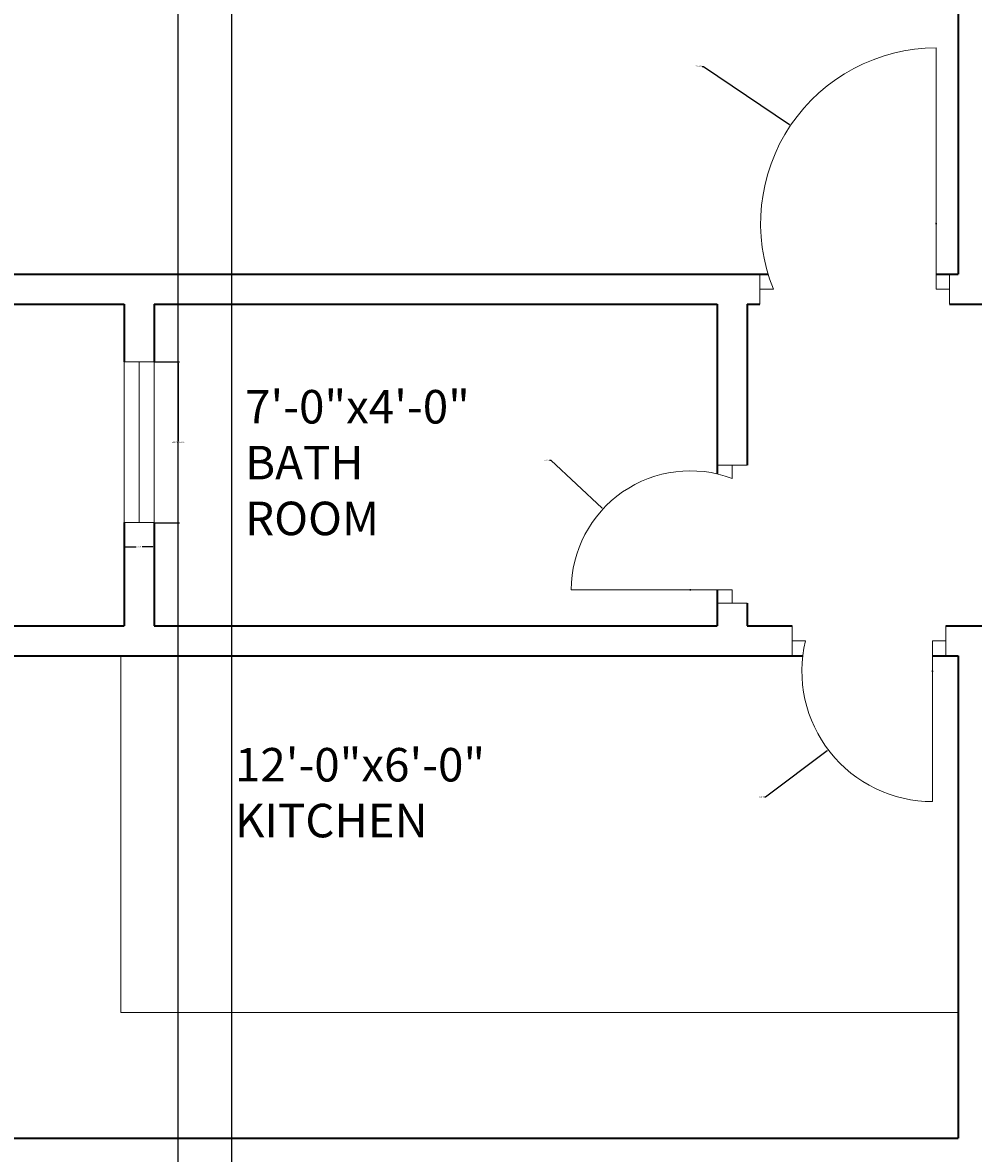
# Model space of a CAD drawing. Units: inches. Extents: x 2163 to 2982, y 1024 to 2288.
# Tile 11 of 22: x 2306 to 2448, y 1885 to 2054. Entities that reach past the tile are written whole.
import ezdxf

# ---------------------------------------------------------------- set-up
doc = ezdxf.new("R2010")
doc.units = ezdxf.units.IN
for name, color, linetype, lineweight in [('A-ANNO-DIMS', 2, 'Continuous', 18), ('A-AREA-IDEN', 7, 'Continuous', 18), ('A-DOOR', 11, 'Continuous', 18), ('A-FLOR-FIXT', 9, 'Continuous', 18), ('A-GLAZ', 161, 'Continuous', 18), ('A-WALL', 7, 'Continuous', 35)]:
    doc.layers.add(name, color=color, linetype=linetype, lineweight=lineweight)
doc.styles.get("Standard").update_dxf_attribs({"font": 'arial.ttf'})
doc.dimstyles.get("Standard").update_dxf_attribs({"dimtxt": 0.18, "dimasz": 0.18, "dimexe": 0.18, "dimexo": 0.0625, "dimgap": 0.09, "dimtad": 0, "dimtih": 1, "dimtoh": 1, "dimdec": 4, "dimzin": 0, "dimdsep": 46, "dimtxsty": 'Standard', "dimcen": 0.09, "dimadec": 0, "dimazin": 0, "dimtfac": 1, "dimtdec": 4, "dimtofl": 0, "dimtmove": 0, "dimatfit": 3, "dimfxl": 1, "dimtolj": 1, "dimtzin": 0, "dimarcsym": 0})

# ---------------------------------------------------------------- blocks, each defined once
blk = doc.blocks.new('WIN-24')
for p, q in [((0, 24), (4.5, 24)), ((0, 24), (0, 0)), ((4.5, 24), (2.25, 24)), ((2.25, 24), (2.25, 0)), ((4.5, 24), (4.5, 0)), ((2.25, 0), (0, 0)), ((0, 0), (4.5, 0))]:
    blk.add_line(p, q)
blk = doc.blocks.new('*D11')
at = {"layer": 'A-ANNO-DIMS', "color": 0, "lineweight": -2, "transparency": 16777216}
for p, q in [((2325.9, 2003.16), (2329.62, 2003.16)), ((2329.44, 2002.98), (2329.44, 1991.35)), ((2329.44, 1979.34), (2329.44, 1990.98)), ((2325.9, 1979.16), (2329.62, 1979.16))]:
    blk.add_line(p, q, dxfattribs=at)
at = {"layer": 'A-ANNO-DIMS', "color": 0, "transparency": 16777216}
for points in [[(2329.41, 2002.98), (2329.47, 2002.98), (2329.44, 2003.16)], [(2329.41, 1979.34), (2329.47, 1979.34), (2329.44, 1979.16)]]:
    blk.add_solid(points, dxfattribs=at)
at = {"layer": 'Defpoints', "color": 0, "transparency": 16777216}
for p in [(2325.84, 2003.16), (2329.44, 2003.16), (2325.84, 1979.16)]:
    blk.add_point(p, dxfattribs=at)
at = {"layer": 'A-ANNO-DIMS', "color": 0, "transparency": 16777216, "insert": (2329.44, 1991.16), "char_height": 0.18, "attachment_point": 5}
blk.add_mtext('\\A1;WINDOW 24 TYP.', dxfattribs=at)
blk = doc.blocks.new('*D12')
at = {"layer": 'A-ANNO-DIMS', "color": 0, "lineweight": -2, "transparency": 16777216}
for p, q in [((2321.34, 1979.1), (2321.34, 1975.38)), ((2325.84, 1979.1), (2325.84, 1975.38)), ((2321.52, 1975.56), (2323.13, 1975.56)), ((2325.66, 1975.56), (2324.05, 1975.56))]:
    blk.add_line(p, q, dxfattribs=at)
at = {"layer": 'A-ANNO-DIMS', "color": 0, "transparency": 16777216}
for points in [[(2321.52, 1975.59), (2321.52, 1975.53), (2321.34, 1975.56)], [(2325.66, 1975.59), (2325.66, 1975.53), (2325.84, 1975.56)]]:
    blk.add_solid(points, dxfattribs=at)
at = {"layer": 'Defpoints', "color": 0, "transparency": 16777216}
for p in [(2321.34, 1979.16), (2325.84, 1979.16), (2325.84, 1975.56)]:
    blk.add_point(p, dxfattribs=at)
at = {"layer": 'A-ANNO-DIMS', "color": 0, "transparency": 16777216, "insert": (2323.59, 1975.56), "char_height": 0.18, "attachment_point": 5}
blk.add_mtext('\\A1;5 TYP.', dxfattribs=at)
blk = doc.blocks.new('*D29')
at = {"layer": 'A-ANNO-DIMS', "color": 0, "lineweight": -2, "transparency": 16777216}
for p, q in [((2285.34, 1738.83), (2285.34, 2288.1)), ((2285.52, 2287.92), (2576.05, 2287.92)), ((2867.16, 2287.92), (2576.63, 2287.92)), ((2867.34, 2229.33), (2867.34, 2288.1))]:
    blk.add_line(p, q, dxfattribs=at)
at = {"layer": 'A-ANNO-DIMS', "color": 0, "transparency": 16777216}
for points in [[(2285.52, 2287.95), (2285.52, 2287.89), (2285.34, 2287.92)], [(2867.16, 2287.95), (2867.16, 2287.89), (2867.34, 2287.92)]]:
    blk.add_solid(points, dxfattribs=at)
at = {"layer": 'Defpoints', "color": 0, "transparency": 16777216}
for p in [(2867.34, 2287.92), (2867.34, 2229.27), (2285.34, 1738.77)]:
    blk.add_point(p, dxfattribs=at)
at = {"layer": 'A-ANNO-DIMS', "color": 0, "transparency": 16777216, "insert": (2576.34, 2287.92), "char_height": 0.18, "attachment_point": 5}
blk.add_mtext('\\A1;582', dxfattribs=at)
blk = doc.blocks.new('*D38')
at = {"layer": 'A-ANNO-DIMS', "color": 0, "lineweight": -2, "transparency": 16777216}
for p, q in [((2329.44, 1734.33), (2329.44, 2288.1)), ((2329.62, 2287.92), (2333.29, 2287.92)), ((2337.26, 2287.92), (2333.59, 2287.92)), ((2337.44, 1734.33), (2337.44, 2288.1))]:
    blk.add_line(p, q, dxfattribs=at)
at = {"layer": 'A-ANNO-DIMS', "color": 0, "transparency": 16777216}
for points in [[(2329.62, 2287.95), (2329.62, 2287.89), (2329.44, 2287.92)], [(2337.26, 2287.95), (2337.26, 2287.89), (2337.44, 2287.92)]]:
    blk.add_solid(points, dxfattribs=at)
at = {"layer": 'Defpoints', "color": 0, "transparency": 16777216}
for p in [(2337.44, 2287.92), (2329.44, 1734.27), (2337.44, 1734.27)]:
    blk.add_point(p, dxfattribs=at)
at = {"layer": 'A-ANNO-DIMS', "color": 0, "transparency": 16777216, "insert": (2333.44, 2287.92), "char_height": 0.18, "attachment_point": 5}
blk.add_mtext('\\A1;8', dxfattribs=at)
blk = doc.blocks.new('*D53')
at = {"layer": 'A-ANNO-DIMS', "color": 0, "lineweight": -2, "transparency": 16777216}
for p, q in [((2407.61, 2047.27), (2407.79, 2047.27)), ((2407.79, 2047.27), (2420.67, 2038.58)), ((2442.45, 2023.82), (2442.63, 2023.82)), ((2442.54, 2023.73), (2442.54, 2023.91))]:
    blk.add_line(p, q, dxfattribs=at)
at = {"layer": 'A-ANNO-DIMS', "color": 0, "transparency": 16777216}
blk.add_solid([(2420.69, 2038.6), (2420.66, 2038.55), (2420.82, 2038.48)], dxfattribs=at)
at = {"layer": 'Defpoints', "color": 0, "transparency": 16777216}
for p in [(2420.82, 2038.48), (2442.54, 2023.82)]:
    blk.add_point(p, dxfattribs=at)
at = {"layer": 'A-ANNO-DIMS', "color": 0, "transparency": 16777216, "insert": (2407.06, 2047.27), "char_height": 0.18, "attachment_point": 5}
blk.add_mtext('\\A1;R26.203', dxfattribs=at)
blk = doc.blocks.new('*D69')
at = {"layer": 'A-ANNO-DIMS', "color": 0, "lineweight": -2, "transparency": 16777216}
for p, q in [((2384.85, 1988.48), (2385.03, 1988.48)), ((2385.03, 1988.48), (2392.7, 1981.35)), ((2405.76, 1969.14), (2405.94, 1969.14)), ((2405.85, 1969.05), (2405.85, 1969.23))]:
    blk.add_line(p, q, dxfattribs=at)
at = {"layer": 'A-ANNO-DIMS', "color": 0, "transparency": 16777216}
blk.add_solid([(2392.72, 1981.37), (2392.68, 1981.33), (2392.83, 1981.23)], dxfattribs=at)
at = {"layer": 'Defpoints', "color": 0, "transparency": 16777216}
for p in [(2392.83, 1981.23), (2405.85, 1969.14)]:
    blk.add_point(p, dxfattribs=at)
at = {"layer": 'A-ANNO-DIMS', "color": 0, "transparency": 16777216, "insert": (2384.37, 1988.48), "char_height": 0.18, "attachment_point": 5}
blk.add_mtext('\\A1;R17.76', dxfattribs=at)
blk = doc.blocks.new('*D71')
at = {"layer": 'A-ANNO-DIMS', "color": 0, "lineweight": -2, "transparency": 16777216}
for p, q in [((2441.91, 1957.02), (2442.09, 1957.02)), ((2442, 1956.93), (2442, 1957.11)), ((2417.09, 1938.22), (2426.29, 1945.16)), ((2416.91, 1938.22), (2417.09, 1938.22))]:
    blk.add_line(p, q, dxfattribs=at)
at = {"layer": 'A-ANNO-DIMS', "color": 0, "transparency": 16777216}
blk.add_solid([(2426.27, 1945.19), (2426.31, 1945.14), (2426.43, 1945.27)], dxfattribs=at)
at = {"layer": 'Defpoints', "color": 0, "transparency": 16777216}
for p in [(2442, 1957.02), (2426.43, 1945.27)]:
    blk.add_point(p, dxfattribs=at)
at = {"layer": 'A-ANNO-DIMS', "color": 0, "transparency": 16777216, "insert": (2416.5, 1938.22), "char_height": 0.18, "attachment_point": 5}
blk.add_mtext('\\A1;R19.5', dxfattribs=at)

msp = doc.modelspace()

# ---------------------------------------------------------------- linework, layer by layer
at = {"layer": 'A-DOOR'}
for p, q in [((2442.5397, 2014.0188), (2442.5397, 2050.0188)), ((2416.237, 2016.2688), (2416.237, 2011.7688)), ((2444.5397, 2016.2688), (2444.5397, 2011.7688)), ((2416.237, 2011.7688), (2416.237, 2014.0188)), ((2416.237, 2014.0188), (2418.237, 2014.0188)), ((2444.5397, 2014.0188), (2442.5397, 2014.0188)), ((2444.5397, 2011.7688), (2444.5397, 2014.0188)), ((2409.8389, 1987.7688), (2414.3389, 1987.7688)), ((2414.3389, 1987.7688), (2412.0889, 1987.7688)), ((2412.0889, 1987.7688), (2412.0889, 1985.7688)), ((2412.0889, 1969.1408), (2388.0889, 1969.1408)), ((2412.0889, 1967.1408), (2412.0889, 1969.1408)), ((2409.8389, 1967.1408), (2414.3389, 1967.1408)), ((2414.3389, 1967.1408), (2412.0889, 1967.1408)), ((2421.0228, 1963.7688), (2421.0228, 1959.2688)), ((2443.9958, 1959.2688), (2443.9958, 1963.7688)), ((2443.9958, 1963.7688), (2443.9958, 1961.5188)), ((2421.0228, 1959.2688), (2421.0228, 1961.5188)), ((2421.0228, 1961.5188), (2423.0228, 1961.5188)), ((2443.9958, 1961.5188), (2441.9958, 1961.5188)), ((2441.9958, 1961.5188), (2441.9958, 1937.5188))]:
    msp.add_line(p, q, dxfattribs=at)
for centre, radius, start, end in [((2442.5397, 2023.8158), 26.2031, 90, 201.955351), ((2405.8491, 1969.1408), 17.7602, 69.431033, 180), ((2441.9958, 1957.0183), 19.4995, 166.655762, 270)]:
    msp.add_arc(centre, radius, start, end, dxfattribs=at)
at = {"layer": 'A-FLOR-FIXT'}
for p, q in [((2320.8872, 1906.0638), (2320.8872, 1959.2688)), ((2445.8389, 1906.0638), (2320.8872, 1906.0638))]:
    msp.add_line(p, q, dxfattribs=at)
at = {"layer": 'A-WALL'}
for p, q in [((2445.8389, 2172.2688), (2445.8389, 2016.2688)), ((2301.8389, 2016.2688), (2417.447, 2016.2688)), ((2442.5397, 2016.2688), (2445.8389, 2016.2688)), ((2297.3389, 2011.7688), (2321.3389, 2011.7688)), ((2321.3389, 2011.7688), (2321.3389, 2003.1644)), ((2325.8389, 2011.7688), (2325.8389, 2003.1644)), ((2325.8389, 2011.7688), (2409.8389, 2011.7688)), ((2409.8389, 2011.7688), (2409.8389, 1986.4471)), ((2414.3389, 2011.7688), (2414.3389, 1987.7688)), ((2414.3389, 2011.7688), (2416.237, 2011.7688)), ((2444.5397, 2011.7688), (2450.3389, 2011.7688)), ((2321.3389, 1979.1644), (2321.3389, 1963.7688)), ((2325.8389, 1979.1644), (2325.8389, 1963.7688)), ((2409.8389, 1969.1408), (2409.8389, 1963.7688)), ((2414.3389, 1967.1408), (2414.3389, 1963.7688)), ((2297.3389, 1963.7688), (2321.3389, 1963.7688)), ((2325.8389, 1963.7688), (2409.8389, 1963.7688)), ((2414.3389, 1963.7688), (2421.0228, 1963.7688)), ((2443.9958, 1963.7688), (2450.3389, 1963.7688)), ((2301.8389, 1959.2688), (2422.6267, 1959.2688)), ((2441.9958, 1959.2688), (2445.8389, 1959.2688)), ((2445.8389, 1959.2688), (2445.8389, 1887.2688)), ((2301.8389, 1887.2688), (2445.8389, 1887.2688))]:
    msp.add_line(p, q, dxfattribs=at)

# ---------------------------------------------------------------- block references
at = {"layer": 'A-GLAZ'}
msp.add_blockref('WIN-24', (2321.339, 1979.1648), dxfattribs=at)

# ---------------------------------------------------------------- texts
at = {"layer": 'A-AREA-IDEN', "char_height": 5, "attachment_point": 1}
for s, width, insert in [('7\'-0"x4\'-0"\\PBATH ROOM', 38.368739, (2339.412, 1998.9635)), ('12\'-0"x6\'-0"\\PKITCHEN', 71.179522, (2337.9016, 1945.5304))]:
    msp.add_mtext_dynamic_manual_height_columns(s, width=width, gutter_width=12.5, heights=[0], dxfattribs=dict(at, insert=insert))

# ---------------------------------------------------------------- dimensions: what is measured, and where the dimension line sits
at = {"layer": 'A-ANNO-DIMS'}
for base, p1, p2, picture, middle in [((2867.3389, 2287.9188), (2285.3389, 1738.7688), (2867.3389, 2229.2688), '*D29', (2576.3389, 2287.9188)), ((2337.4434, 2287.9188), (2329.4434, 1734.2688), (2337.4434, 1734.2688), '*D38', (2333.4434, 2287.9188))]:
    dim = msp.add_linear_dim(base=base, p1=p1, p2=p2, dimstyle='Standard', override={"dimdec": 0, "dimlfac": 1, "dimrnd": 0, "dimzin": 0, "dimdsep": 46, "dimlunit": 2}, dxfattribs=at)
    dim.commit()
    dim.dimension.update_dxf_attribs({"geometry": picture, "text_midpoint": middle})
for center, mpoint, override, picture, middle in [((2442.5397, 2023.8158), (2420.8221, 2038.4769), {"dimdec": 3, "dimlfac": 1, "dimrnd": 0, "dimzin": 0, "dimdsep": 46, "dimlunit": 2}, '*D53', (2407.0618, 2047.2736)), ((2405.8491, 1969.1408), (2392.8342, 1981.2254), {"dimdec": 2, "dimlfac": 1, "dimrnd": 0, "dimzin": 0, "dimdsep": 46, "dimlunit": 2}, '*D69', (2384.3655, 1988.4762)), ((2441.9958, 1957.0183), (2426.4319, 1945.2712), {"dimdec": 1, "dimlfac": 1, "dimrnd": 0, "dimzin": 0, "dimdsep": 46, "dimlunit": 2}, '*D71', (2416.503, 1938.223))]:
    dim = msp.add_radius_dim(center=center, mpoint=mpoint, dimstyle='Standard', override=override, dxfattribs=at)
    dim.commit()
    dim.dimension.update_dxf_attribs({"geometry": picture, "text_midpoint": middle, "dimtype": 164})
dim = msp.add_linear_dim(base=(2329.4389, 2003.1644), p1=(2325.8389, 1979.1644), p2=(2325.8389, 2003.1644), angle=90, text='WINDOW <> TYP.', dimstyle='Standard', override={"dimdec": 0, "dimlfac": 1, "dimrnd": 0, "dimzin": 0, "dimdsep": 46, "dimlunit": 2}, dxfattribs=at)
dim.commit()
dim.dimension.update_dxf_attribs({"geometry": '*D11', "text_midpoint": (2329.4389, 1991.1644)})
dim = msp.add_linear_dim(base=(2325.8389150341, 1975.564374433), p1=(2321.3389150341, 1979.164374433), p2=(2325.8389150341, 1979.164374433), text='<> TYP.', dimstyle='Standard', override={"dimdec": 0, "dimlfac": 1, "dimrnd": 0, "dimzin": 0, "dimdsep": 46, "dimlunit": 2}, dxfattribs=at)
dim.commit()
dim.dimension.update_dxf_attribs({"geometry": '*D12', "text_midpoint": (2323.5889150341, 1975.564374433)})

doc.saveas('drawing.dxf')
